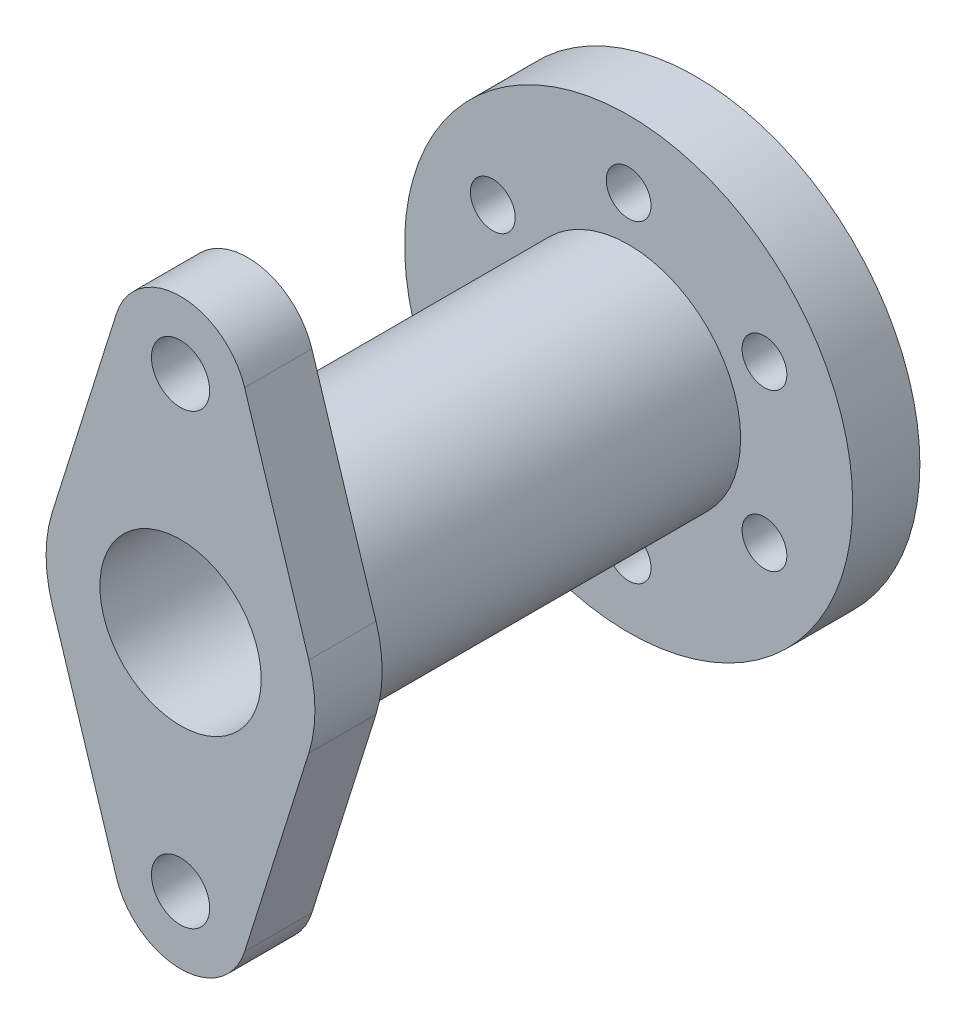
ISO-10303-21;
HEADER;
FILE_DESCRIPTION(('STEP AP214'),'2;1');
FILE_NAME('part.step','',(''),(''),'','','');
FILE_SCHEMA(('AUTOMOTIVE_DESIGN { 1 0 10303 214 1 1 1 1 }'));
ENDSEC;
DATA;
#1=APPLICATION_CONTEXT('core data for automotive mechanical design processes');
#2=APPLICATION_PROTOCOL_DEFINITION('international standard','automotive_design',2000,#1);
#3=PRODUCT_CONTEXT('',#1,'mechanical');
#4=PRODUCT('Part','Part','',(#3));
#5=PRODUCT_RELATED_PRODUCT_CATEGORY('part','',(#4));
#6=PRODUCT_DEFINITION_FORMATION('','',#4);
#7=PRODUCT_DEFINITION_CONTEXT('part definition',#1,'design');
#8=PRODUCT_DEFINITION('design','',#6,#7);
#9=PRODUCT_DEFINITION_SHAPE('','',#8);
#10=(LENGTH_UNIT() NAMED_UNIT(*) SI_UNIT(.MILLI.,.METRE.));
#11=(NAMED_UNIT(*) PLANE_ANGLE_UNIT() SI_UNIT($,.RADIAN.));
#12=(NAMED_UNIT(*) SI_UNIT($,.STERADIAN.) SOLID_ANGLE_UNIT());
#13=UNCERTAINTY_MEASURE_WITH_UNIT(LENGTH_MEASURE(1.E-05),#10,'distance_accuracy_value','');
#14=(GEOMETRIC_REPRESENTATION_CONTEXT(3) GLOBAL_UNCERTAINTY_ASSIGNED_CONTEXT((#13)) GLOBAL_UNIT_ASSIGNED_CONTEXT((#10,
#11,#12)) REPRESENTATION_CONTEXT('',''));
#15=CARTESIAN_POINT('',(0.,0.,0.));
#16=DIRECTION('',(0.,0.,1.));
#17=DIRECTION('',(1.,0.,0.));
#18=AXIS2_PLACEMENT_3D('',#15,#16,#17);
#19=CARTESIAN_POINT('',(0.,0.,15.));
#20=DIRECTION('',(0.,0.,-1.));
#21=DIRECTION('',(-1.,0.,0.));
#22=AXIS2_PLACEMENT_3D('',#19,#20,#21);
#23=CYLINDRICAL_SURFACE('',#22,50.);
#24=CARTESIAN_POINT('',(0.,0.,15.));
#25=DIRECTION('',(0.,0.,1.));
#26=DIRECTION('',(1.,0.,0.));
#27=AXIS2_PLACEMENT_3D('',#24,#25,#26);
#28=CIRCLE('',#27,50.);
#29=CARTESIAN_POINT('',(50.,0.,15.));
#30=VERTEX_POINT('',#29);
#31=EDGE_CURVE('E11',#30,#30,#28,.T.);
#32=ORIENTED_EDGE('',*,*,#31,.F.);
#33=EDGE_LOOP('',(#32));
#34=FACE_BOUND('',#33,.T.);
#35=CARTESIAN_POINT('',(0.,0.,0.));
#36=DIRECTION('',(0.,0.,1.));
#37=DIRECTION('',(1.,0.,0.));
#38=AXIS2_PLACEMENT_3D('',#35,#36,#37);
#39=CIRCLE('',#38,50.);
#40=CARTESIAN_POINT('',(50.,0.,0.));
#41=VERTEX_POINT('',#40);
#42=EDGE_CURVE('E48',#41,#41,#39,.T.);
#43=ORIENTED_EDGE('',*,*,#42,.T.);
#44=EDGE_LOOP('',(#43));
#45=FACE_BOUND('',#44,.T.);
#46=ADVANCED_FACE('F44',(#34,#45),#23,.T.);
#47=CARTESIAN_POINT('',(0.,0.,15.));
#48=DIRECTION('',(0.,0.,1.));
#49=DIRECTION('',(1.,0.,0.));
#50=AXIS2_PLACEMENT_3D('',#47,#48,#49);
#51=PLANE('',#50);
#52=CARTESIAN_POINT('',(0.,0.,15.));
#53=DIRECTION('',(0.,0.,1.));
#54=DIRECTION('',(1.,0.,0.));
#55=AXIS2_PLACEMENT_3D('',#52,#53,#54);
#56=CIRCLE('',#55,25.);
#57=CARTESIAN_POINT('',(25.,0.,15.));
#58=VERTEX_POINT('',#57);
#59=EDGE_CURVE('E175',#58,#58,#56,.T.);
#60=ORIENTED_EDGE('',*,*,#59,.F.);
#61=EDGE_LOOP('',(#60));
#62=FACE_BOUND('',#61,.T.);
#63=CARTESIAN_POINT('',(0.,-35.,15.));
#64=DIRECTION('',(0.,0.,1.));
#65=DIRECTION('',(1.,0.,0.));
#66=AXIS2_PLACEMENT_3D('',#63,#64,#65);
#67=CIRCLE('',#66,5.);
#68=CARTESIAN_POINT('',(5.,-35.,15.));
#69=VERTEX_POINT('',#68);
#70=EDGE_CURVE('E176',#69,#69,#67,.T.);
#71=ORIENTED_EDGE('',*,*,#70,.F.);
#72=EDGE_LOOP('',(#71));
#73=FACE_BOUND('',#72,.T.);
#74=CARTESIAN_POINT('',(30.3108891324553,-17.5000000000001,15.));
#75=DIRECTION('',(0.,0.,1.));
#76=DIRECTION('',(1.,0.,0.));
#77=AXIS2_PLACEMENT_3D('',#74,#75,#76);
#78=CIRCLE('',#77,5.00000000000004);
#79=CARTESIAN_POINT('',(35.3108891324554,-17.5000000000001,15.));
#80=VERTEX_POINT('',#79);
#81=EDGE_CURVE('E201',#80,#80,#78,.T.);
#82=ORIENTED_EDGE('',*,*,#81,.F.);
#83=EDGE_LOOP('',(#82));
#84=FACE_BOUND('',#83,.T.);
#85=CARTESIAN_POINT('',(-30.3108891324553,-17.5,15.));
#86=DIRECTION('',(0.,0.,1.));
#87=DIRECTION('',(1.,0.,0.));
#88=AXIS2_PLACEMENT_3D('',#85,#86,#87);
#89=CIRCLE('',#88,5.);
#90=CARTESIAN_POINT('',(-25.3108891324553,-17.5,15.));
#91=VERTEX_POINT('',#90);
#92=EDGE_CURVE('E192',#91,#91,#89,.T.);
#93=ORIENTED_EDGE('',*,*,#92,.F.);
#94=EDGE_LOOP('',(#93));
#95=FACE_BOUND('',#94,.T.);
#96=CARTESIAN_POINT('',(30.3108891324553,17.5,15.));
#97=DIRECTION('',(0.,0.,1.));
#98=DIRECTION('',(1.,0.,0.));
#99=AXIS2_PLACEMENT_3D('',#96,#97,#98);
#100=CIRCLE('',#99,5.);
#101=CARTESIAN_POINT('',(35.3108891324553,17.5,15.));
#102=VERTEX_POINT('',#101);
#103=EDGE_CURVE('E186',#102,#102,#100,.T.);
#104=ORIENTED_EDGE('',*,*,#103,.F.);
#105=EDGE_LOOP('',(#104));
#106=FACE_BOUND('',#105,.T.);
#107=CARTESIAN_POINT('',(0.,35.,15.));
#108=DIRECTION('',(0.,0.,1.));
#109=DIRECTION('',(1.,0.,0.));
#110=AXIS2_PLACEMENT_3D('',#107,#108,#109);
#111=CIRCLE('',#110,5.);
#112=CARTESIAN_POINT('',(5.,35.,15.));
#113=VERTEX_POINT('',#112);
#114=EDGE_CURVE('E182',#113,#113,#111,.T.);
#115=ORIENTED_EDGE('',*,*,#114,.F.);
#116=EDGE_LOOP('',(#115));
#117=FACE_BOUND('',#116,.T.);
#118=CARTESIAN_POINT('',(-30.3108891324553,17.5000000000001,15.));
#119=DIRECTION('',(0.,0.,1.));
#120=DIRECTION('',(1.,0.,0.));
#121=AXIS2_PLACEMENT_3D('',#118,#119,#120);
#122=CIRCLE('',#121,4.99999999999997);
#123=CARTESIAN_POINT('',(-25.3108891324554,17.5000000000001,15.));
#124=VERTEX_POINT('',#123);
#125=EDGE_CURVE('E185',#124,#124,#122,.T.);
#126=ORIENTED_EDGE('',*,*,#125,.F.);
#127=EDGE_LOOP('',(#126));
#128=FACE_BOUND('',#127,.T.);
#129=ORIENTED_EDGE('',*,*,#31,.T.);
#130=EDGE_LOOP('',(#129));
#131=FACE_BOUND('',#130,.T.);
#132=ADVANCED_FACE('F220',(#62,#73,#84,#95,#106,#117,#128,#131),#51,.T.);
#133=CARTESIAN_POINT('',(0.,0.,0.));
#134=DIRECTION('',(0.,0.,1.));
#135=DIRECTION('',(1.,0.,0.));
#136=AXIS2_PLACEMENT_3D('',#133,#134,#135);
#137=PLANE('',#136);
#138=CARTESIAN_POINT('',(0.,0.,0.));
#139=DIRECTION('',(0.,0.,1.));
#140=DIRECTION('',(1.,0.,0.));
#141=AXIS2_PLACEMENT_3D('',#138,#139,#140);
#142=CIRCLE('',#141,14.);
#143=CARTESIAN_POINT('',(14.,0.,0.));
#144=VERTEX_POINT('',#143);
#145=EDGE_CURVE('E318',#144,#144,#142,.T.);
#146=ORIENTED_EDGE('',*,*,#145,.T.);
#147=EDGE_LOOP('',(#146));
#148=FACE_BOUND('',#147,.T.);
#149=CARTESIAN_POINT('',(0.,-35.,0.));
#150=DIRECTION('',(0.,0.,1.));
#151=DIRECTION('',(1.,0.,0.));
#152=AXIS2_PLACEMENT_3D('',#149,#150,#151);
#153=CIRCLE('',#152,5.);
#154=CARTESIAN_POINT('',(5.,-35.,0.));
#155=VERTEX_POINT('',#154);
#156=EDGE_CURVE('E202',#155,#155,#153,.T.);
#157=ORIENTED_EDGE('',*,*,#156,.T.);
#158=EDGE_LOOP('',(#157));
#159=FACE_BOUND('',#158,.T.);
#160=CARTESIAN_POINT('',(30.3108891324553,-17.5000000000001,0.));
#161=DIRECTION('',(0.,0.,1.));
#162=DIRECTION('',(1.,0.,0.));
#163=AXIS2_PLACEMENT_3D('',#160,#161,#162);
#164=CIRCLE('',#163,5.00000000000004);
#165=CARTESIAN_POINT('',(35.3108891324554,-17.5000000000001,0.));
#166=VERTEX_POINT('',#165);
#167=EDGE_CURVE('E196',#166,#166,#164,.T.);
#168=ORIENTED_EDGE('',*,*,#167,.T.);
#169=EDGE_LOOP('',(#168));
#170=FACE_BOUND('',#169,.T.);
#171=CARTESIAN_POINT('',(-30.3108891324553,-17.5,0.));
#172=DIRECTION('',(0.,0.,1.));
#173=DIRECTION('',(1.,0.,0.));
#174=AXIS2_PLACEMENT_3D('',#171,#172,#173);
#175=CIRCLE('',#174,5.);
#176=CARTESIAN_POINT('',(-25.3108891324553,-17.5,0.));
#177=VERTEX_POINT('',#176);
#178=EDGE_CURVE('E191',#177,#177,#175,.T.);
#179=ORIENTED_EDGE('',*,*,#178,.T.);
#180=EDGE_LOOP('',(#179));
#181=FACE_BOUND('',#180,.T.);
#182=CARTESIAN_POINT('',(30.3108891324553,17.5,0.));
#183=DIRECTION('',(0.,0.,1.));
#184=DIRECTION('',(1.,0.,0.));
#185=AXIS2_PLACEMENT_3D('',#182,#183,#184);
#186=CIRCLE('',#185,5.);
#187=CARTESIAN_POINT('',(35.3108891324553,17.5,0.));
#188=VERTEX_POINT('',#187);
#189=EDGE_CURVE('E187',#188,#188,#186,.T.);
#190=ORIENTED_EDGE('',*,*,#189,.T.);
#191=EDGE_LOOP('',(#190));
#192=FACE_BOUND('',#191,.T.);
#193=CARTESIAN_POINT('',(0.,35.,0.));
#194=DIRECTION('',(0.,0.,1.));
#195=DIRECTION('',(1.,0.,0.));
#196=AXIS2_PLACEMENT_3D('',#193,#194,#195);
#197=CIRCLE('',#196,5.);
#198=CARTESIAN_POINT('',(5.,35.,0.));
#199=VERTEX_POINT('',#198);
#200=EDGE_CURVE('E177',#199,#199,#197,.T.);
#201=ORIENTED_EDGE('',*,*,#200,.T.);
#202=EDGE_LOOP('',(#201));
#203=FACE_BOUND('',#202,.T.);
#204=CARTESIAN_POINT('',(-30.3108891324553,17.5000000000001,0.));
#205=DIRECTION('',(0.,0.,1.));
#206=DIRECTION('',(1.,0.,0.));
#207=AXIS2_PLACEMENT_3D('',#204,#205,#206);
#208=CIRCLE('',#207,4.99999999999997);
#209=CARTESIAN_POINT('',(-25.3108891324554,17.5000000000001,0.));
#210=VERTEX_POINT('',#209);
#211=EDGE_CURVE('E209',#210,#210,#208,.T.);
#212=ORIENTED_EDGE('',*,*,#211,.T.);
#213=EDGE_LOOP('',(#212));
#214=FACE_BOUND('',#213,.T.);
#215=ORIENTED_EDGE('',*,*,#42,.F.);
#216=EDGE_LOOP('',(#215));
#217=FACE_BOUND('',#216,.T.);
#218=ADVANCED_FACE('F217',(#148,#159,#170,#181,#192,#203,#214,#217),#137,.F.);
#219=CARTESIAN_POINT('',(-30.3108891324553,17.5000000000001,0.));
#220=DIRECTION('',(0.,0.,1.));
#221=DIRECTION('',(1.,0.,0.));
#222=AXIS2_PLACEMENT_3D('',#219,#220,#221);
#223=CYLINDRICAL_SURFACE('',#222,4.99999999999997);
#224=ORIENTED_EDGE('',*,*,#211,.F.);
#225=EDGE_LOOP('',(#224));
#226=FACE_BOUND('',#225,.T.);
#227=ORIENTED_EDGE('',*,*,#125,.T.);
#228=EDGE_LOOP('',(#227));
#229=FACE_BOUND('',#228,.T.);
#230=ADVANCED_FACE('F212',(#226,#229),#223,.F.);
#231=CARTESIAN_POINT('',(0.,35.,0.));
#232=DIRECTION('',(0.,0.,1.));
#233=DIRECTION('',(1.,0.,0.));
#234=AXIS2_PLACEMENT_3D('',#231,#232,#233);
#235=CYLINDRICAL_SURFACE('',#234,5.);
#236=ORIENTED_EDGE('',*,*,#200,.F.);
#237=EDGE_LOOP('',(#236));
#238=FACE_BOUND('',#237,.T.);
#239=ORIENTED_EDGE('',*,*,#114,.T.);
#240=EDGE_LOOP('',(#239));
#241=FACE_BOUND('',#240,.T.);
#242=ADVANCED_FACE('F236',(#238,#241),#235,.F.);
#243=CARTESIAN_POINT('',(30.3108891324553,17.5,0.));
#244=DIRECTION('',(0.,0.,1.));
#245=DIRECTION('',(1.,0.,0.));
#246=AXIS2_PLACEMENT_3D('',#243,#244,#245);
#247=CYLINDRICAL_SURFACE('',#246,5.);
#248=ORIENTED_EDGE('',*,*,#189,.F.);
#249=EDGE_LOOP('',(#248));
#250=FACE_BOUND('',#249,.T.);
#251=ORIENTED_EDGE('',*,*,#103,.T.);
#252=EDGE_LOOP('',(#251));
#253=FACE_BOUND('',#252,.T.);
#254=ADVANCED_FACE('F251',(#250,#253),#247,.F.);
#255=CARTESIAN_POINT('',(-30.3108891324553,-17.5,0.));
#256=DIRECTION('',(0.,0.,1.));
#257=DIRECTION('',(1.,0.,0.));
#258=AXIS2_PLACEMENT_3D('',#255,#256,#257);
#259=CYLINDRICAL_SURFACE('',#258,5.);
#260=ORIENTED_EDGE('',*,*,#178,.F.);
#261=EDGE_LOOP('',(#260));
#262=FACE_BOUND('',#261,.T.);
#263=ORIENTED_EDGE('',*,*,#92,.T.);
#264=EDGE_LOOP('',(#263));
#265=FACE_BOUND('',#264,.T.);
#266=ADVANCED_FACE('F249',(#262,#265),#259,.F.);
#267=CARTESIAN_POINT('',(30.3108891324553,-17.5000000000001,0.));
#268=DIRECTION('',(0.,0.,1.));
#269=DIRECTION('',(1.,0.,0.));
#270=AXIS2_PLACEMENT_3D('',#267,#268,#269);
#271=CYLINDRICAL_SURFACE('',#270,5.00000000000004);
#272=ORIENTED_EDGE('',*,*,#167,.F.);
#273=EDGE_LOOP('',(#272));
#274=FACE_BOUND('',#273,.T.);
#275=ORIENTED_EDGE('',*,*,#81,.T.);
#276=EDGE_LOOP('',(#275));
#277=FACE_BOUND('',#276,.T.);
#278=ADVANCED_FACE('F246',(#274,#277),#271,.F.);
#279=CARTESIAN_POINT('',(0.,-35.,0.));
#280=DIRECTION('',(0.,0.,1.));
#281=DIRECTION('',(1.,0.,0.));
#282=AXIS2_PLACEMENT_3D('',#279,#280,#281);
#283=CYLINDRICAL_SURFACE('',#282,5.);
#284=ORIENTED_EDGE('',*,*,#156,.F.);
#285=EDGE_LOOP('',(#284));
#286=FACE_BOUND('',#285,.T.);
#287=ORIENTED_EDGE('',*,*,#70,.T.);
#288=EDGE_LOOP('',(#287));
#289=FACE_BOUND('',#288,.T.);
#290=ADVANCED_FACE('F245',(#286,#289),#283,.F.);
#291=CARTESIAN_POINT('',(0.,0.,100.));
#292=DIRECTION('',(0.,0.,-1.));
#293=DIRECTION('',(-1.,0.,0.));
#294=AXIS2_PLACEMENT_3D('',#291,#292,#293);
#295=CYLINDRICAL_SURFACE('',#294,25.);
#296=CARTESIAN_POINT('',(0.,0.,100.));
#297=DIRECTION('',(0.,0.,1.));
#298=DIRECTION('',(1.,0.,0.));
#299=AXIS2_PLACEMENT_3D('',#296,#297,#298);
#300=CIRCLE('',#299,25.);
#301=CARTESIAN_POINT('',(25.,0.,100.));
#302=VERTEX_POINT('',#301);
#303=EDGE_CURVE('E173',#302,#302,#300,.T.);
#304=ORIENTED_EDGE('',*,*,#303,.F.);
#305=EDGE_LOOP('',(#304));
#306=FACE_BOUND('',#305,.T.);
#307=ORIENTED_EDGE('',*,*,#59,.T.);
#308=EDGE_LOOP('',(#307));
#309=FACE_BOUND('',#308,.T.);
#310=ADVANCED_FACE('F244',(#306,#309),#295,.T.);
#311=CARTESIAN_POINT('',(0.,0.,115.));
#312=DIRECTION('',(0.,0.,-1.));
#313=DIRECTION('',(-1.,0.,0.));
#314=AXIS2_PLACEMENT_3D('',#311,#312,#313);
#315=CYLINDRICAL_SURFACE('',#314,30.);
#316=CARTESIAN_POINT('',(0.,0.,100.));
#317=DIRECTION('',(0.,0.,1.));
#318=DIRECTION('',(1.,0.,0.));
#319=AXIS2_PLACEMENT_3D('',#316,#317,#318);
#320=CIRCLE('',#319,30.);
#321=CARTESIAN_POINT('',(-28.6181760425107,8.99999999999249,100.));
#322=VERTEX_POINT('',#321);
#323=CARTESIAN_POINT('',(-28.6181760425107,-8.9999999999925,100.));
#324=VERTEX_POINT('',#323);
#325=EDGE_CURVE('E145',#322,#324,#320,.T.);
#326=ORIENTED_EDGE('',*,*,#325,.T.);
#327=DIRECTION('',(0.,0.,-1.));
#328=VECTOR('',#327,1.);
#329=CARTESIAN_POINT('',(-28.6181760425107,-8.9999999999925,115.));
#330=LINE('',#329,#328);
#331=CARTESIAN_POINT('',(-28.6181760425107,-8.9999999999925,115.));
#332=VERTEX_POINT('',#331);
#333=EDGE_CURVE('E167',#332,#324,#330,.T.);
#334=ORIENTED_EDGE('',*,*,#333,.F.);
#335=CARTESIAN_POINT('',(0.,0.,115.));
#336=DIRECTION('',(0.,0.,1.));
#337=DIRECTION('',(1.,0.,0.));
#338=AXIS2_PLACEMENT_3D('',#335,#336,#337);
#339=CIRCLE('',#338,30.);
#340=CARTESIAN_POINT('',(-28.6181760425107,8.99999999999249,115.));
#341=VERTEX_POINT('',#340);
#342=EDGE_CURVE('E160',#341,#332,#339,.T.);
#343=ORIENTED_EDGE('',*,*,#342,.F.);
#344=DIRECTION('',(0.,0.,-1.));
#345=VECTOR('',#344,1.);
#346=CARTESIAN_POINT('',(-28.6181760425107,8.99999999999249,115.));
#347=LINE('',#346,#345);
#348=EDGE_CURVE('E138',#341,#322,#347,.T.);
#349=ORIENTED_EDGE('',*,*,#348,.T.);
#350=EDGE_LOOP('',(#326,#334,#343,#349));
#351=FACE_BOUND('',#350,.T.);
#352=ADVANCED_FACE('F261',(#351),#315,.T.);
#353=CARTESIAN_POINT('',(-28.6181760425107,-8.9999999999925,115.));
#354=DIRECTION('',(0.953939201417024,0.29999999999975,0.));
#355=DIRECTION('',(-0.29999999999975,0.953939201417024,0.));
#356=AXIS2_PLACEMENT_3D('',#353,#354,#355);
#357=PLANE('',#356);
#358=DIRECTION('',(0.29999999999975,-0.953939201417024,0.));
#359=VECTOR('',#358,1.);
#360=CARTESIAN_POINT('',(-28.6181760425107,-8.9999999999925,100.));
#361=LINE('',#360,#359);
#362=CARTESIAN_POINT('',(-14.3090880212673,-54.5,100.));
#363=VERTEX_POINT('',#362);
#364=EDGE_CURVE('E143',#324,#363,#361,.T.);
#365=ORIENTED_EDGE('',*,*,#364,.T.);
#366=DIRECTION('',(0.,0.,-1.));
#367=VECTOR('',#366,1.);
#368=CARTESIAN_POINT('',(-14.3090880212673,-54.5,115.));
#369=LINE('',#368,#367);
#370=CARTESIAN_POINT('',(-14.3090880212673,-54.5,115.));
#371=VERTEX_POINT('',#370);
#372=EDGE_CURVE('E170',#371,#363,#369,.T.);
#373=ORIENTED_EDGE('',*,*,#372,.F.);
#374=DIRECTION('',(0.29999999999975,-0.953939201417024,0.));
#375=VECTOR('',#374,1.);
#376=CARTESIAN_POINT('',(-28.6181760425107,-8.9999999999925,115.));
#377=LINE('',#376,#375);
#378=EDGE_CURVE('E102',#332,#371,#377,.T.);
#379=ORIENTED_EDGE('',*,*,#378,.F.);
#380=ORIENTED_EDGE('',*,*,#333,.T.);
#381=EDGE_LOOP('',(#365,#373,#379,#380));
#382=FACE_BOUND('',#381,.T.);
#383=ADVANCED_FACE('F270',(#382),#357,.F.);
#384=CARTESIAN_POINT('',(0.,-50.,115.));
#385=DIRECTION('',(0.,0.,-1.));
#386=DIRECTION('',(-1.,0.,0.));
#387=AXIS2_PLACEMENT_3D('',#384,#385,#386);
#388=CYLINDRICAL_SURFACE('',#387,15.0000000000125);
#389=CARTESIAN_POINT('',(0.,-50.,100.));
#390=DIRECTION('',(0.,0.,1.));
#391=DIRECTION('',(1.,0.,0.));
#392=AXIS2_PLACEMENT_3D('',#389,#390,#391);
#393=CIRCLE('',#392,15.0000000000125);
#394=CARTESIAN_POINT('',(14.3090880212673,-54.5,100.));
#395=VERTEX_POINT('',#394);
#396=EDGE_CURVE('E150',#363,#395,#393,.T.);
#397=ORIENTED_EDGE('',*,*,#396,.T.);
#398=DIRECTION('',(0.,0.,-1.));
#399=VECTOR('',#398,1.);
#400=CARTESIAN_POINT('',(14.3090880212673,-54.5,115.));
#401=LINE('',#400,#399);
#402=CARTESIAN_POINT('',(14.3090880212673,-54.5,115.));
#403=VERTEX_POINT('',#402);
#404=EDGE_CURVE('E165',#403,#395,#401,.T.);
#405=ORIENTED_EDGE('',*,*,#404,.F.);
#406=CARTESIAN_POINT('',(0.,-50.,115.));
#407=DIRECTION('',(0.,0.,1.));
#408=DIRECTION('',(1.,0.,0.));
#409=AXIS2_PLACEMENT_3D('',#406,#407,#408);
#410=CIRCLE('',#409,15.0000000000125);
#411=EDGE_CURVE('E348',#371,#403,#410,.T.);
#412=ORIENTED_EDGE('',*,*,#411,.F.);
#413=ORIENTED_EDGE('',*,*,#372,.T.);
#414=EDGE_LOOP('',(#397,#405,#412,#413));
#415=FACE_BOUND('',#414,.T.);
#416=ADVANCED_FACE('F272',(#415),#388,.T.);
#417=CARTESIAN_POINT('',(14.3090880212673,-54.5,115.));
#418=DIRECTION('',(-0.953939201417024,0.29999999999975,0.));
#419=DIRECTION('',(-0.29999999999975,-0.953939201417024,0.));
#420=AXIS2_PLACEMENT_3D('',#417,#418,#419);
#421=PLANE('',#420);
#422=DIRECTION('',(0.29999999999975,0.953939201417024,0.));
#423=VECTOR('',#422,1.);
#424=CARTESIAN_POINT('',(14.3090880212673,-54.5,100.));
#425=LINE('',#424,#423);
#426=CARTESIAN_POINT('',(28.6181760425107,-8.99999999999251,100.));
#427=VERTEX_POINT('',#426);
#428=EDGE_CURVE('E147',#395,#427,#425,.T.);
#429=ORIENTED_EDGE('',*,*,#428,.T.);
#430=DIRECTION('',(0.,0.,-1.));
#431=VECTOR('',#430,1.);
#432=CARTESIAN_POINT('',(28.6181760425107,-8.99999999999251,115.));
#433=LINE('',#432,#431);
#434=CARTESIAN_POINT('',(28.6181760425107,-8.99999999999251,115.));
#435=VERTEX_POINT('',#434);
#436=EDGE_CURVE('E163',#435,#427,#433,.T.);
#437=ORIENTED_EDGE('',*,*,#436,.F.);
#438=DIRECTION('',(0.29999999999975,0.953939201417024,0.));
#439=VECTOR('',#438,1.);
#440=CARTESIAN_POINT('',(14.3090880212673,-54.5,115.));
#441=LINE('',#440,#439);
#442=EDGE_CURVE('E346',#403,#435,#441,.T.);
#443=ORIENTED_EDGE('',*,*,#442,.F.);
#444=ORIENTED_EDGE('',*,*,#404,.T.);
#445=EDGE_LOOP('',(#429,#437,#443,#444));
#446=FACE_BOUND('',#445,.T.);
#447=ADVANCED_FACE('F274',(#446),#421,.F.);
#448=CARTESIAN_POINT('',(0.,0.,115.));
#449=DIRECTION('',(0.,0.,-1.));
#450=DIRECTION('',(-1.,0.,0.));
#451=AXIS2_PLACEMENT_3D('',#448,#449,#450);
#452=CYLINDRICAL_SURFACE('',#451,30.);
#453=CARTESIAN_POINT('',(0.,0.,100.));
#454=DIRECTION('',(0.,0.,1.));
#455=DIRECTION('',(1.,0.,0.));
#456=AXIS2_PLACEMENT_3D('',#453,#454,#455);
#457=CIRCLE('',#456,30.);
#458=CARTESIAN_POINT('',(28.6181760425107,8.99999999999249,100.));
#459=VERTEX_POINT('',#458);
#460=EDGE_CURVE('E155',#427,#459,#457,.T.);
#461=ORIENTED_EDGE('',*,*,#460,.T.);
#462=DIRECTION('',(0.,0.,-1.));
#463=VECTOR('',#462,1.);
#464=CARTESIAN_POINT('',(28.6181760425107,8.99999999999249,115.));
#465=LINE('',#464,#463);
#466=CARTESIAN_POINT('',(28.6181760425107,8.99999999999249,115.));
#467=VERTEX_POINT('',#466);
#468=EDGE_CURVE('E131',#467,#459,#465,.T.);
#469=ORIENTED_EDGE('',*,*,#468,.F.);
#470=CARTESIAN_POINT('',(0.,0.,115.));
#471=DIRECTION('',(0.,0.,1.));
#472=DIRECTION('',(1.,0.,0.));
#473=AXIS2_PLACEMENT_3D('',#470,#471,#472);
#474=CIRCLE('',#473,30.);
#475=EDGE_CURVE('E121',#435,#467,#474,.T.);
#476=ORIENTED_EDGE('',*,*,#475,.F.);
#477=ORIENTED_EDGE('',*,*,#436,.T.);
#478=EDGE_LOOP('',(#461,#469,#476,#477));
#479=FACE_BOUND('',#478,.T.);
#480=ADVANCED_FACE('F280',(#479),#452,.T.);
#481=CARTESIAN_POINT('',(14.3090880212673,54.5,115.));
#482=DIRECTION('',(-0.953939201417024,-0.29999999999975,0.));
#483=DIRECTION('',(0.29999999999975,-0.953939201417024,0.));
#484=AXIS2_PLACEMENT_3D('',#481,#482,#483);
#485=PLANE('',#484);
#486=DIRECTION('',(-0.29999999999975,0.953939201417024,0.));
#487=VECTOR('',#486,1.);
#488=CARTESIAN_POINT('',(14.3090880212673,54.5,100.));
#489=LINE('',#488,#487);
#490=CARTESIAN_POINT('',(14.3090880212673,54.5,100.));
#491=VERTEX_POINT('',#490);
#492=EDGE_CURVE('E135',#459,#491,#489,.T.);
#493=ORIENTED_EDGE('',*,*,#492,.T.);
#494=DIRECTION('',(0.,0.,-1.));
#495=VECTOR('',#494,1.);
#496=CARTESIAN_POINT('',(14.3090880212673,54.5,115.));
#497=LINE('',#496,#495);
#498=CARTESIAN_POINT('',(14.3090880212673,54.5,115.));
#499=VERTEX_POINT('',#498);
#500=EDGE_CURVE('E128',#499,#491,#497,.T.);
#501=ORIENTED_EDGE('',*,*,#500,.F.);
#502=DIRECTION('',(-0.29999999999975,0.953939201417024,0.));
#503=VECTOR('',#502,1.);
#504=CARTESIAN_POINT('',(14.3090880212673,54.5,115.));
#505=LINE('',#504,#503);
#506=EDGE_CURVE('E117',#467,#499,#505,.T.);
#507=ORIENTED_EDGE('',*,*,#506,.F.);
#508=ORIENTED_EDGE('',*,*,#468,.T.);
#509=EDGE_LOOP('',(#493,#501,#507,#508));
#510=FACE_BOUND('',#509,.T.);
#511=ADVANCED_FACE('F127',(#510),#485,.F.);
#512=CARTESIAN_POINT('',(0.,50.,115.));
#513=DIRECTION('',(0.,0.,-1.));
#514=DIRECTION('',(-1.,0.,0.));
#515=AXIS2_PLACEMENT_3D('',#512,#513,#514);
#516=CYLINDRICAL_SURFACE('',#515,15.0000000000125);
#517=CARTESIAN_POINT('',(0.,50.,100.));
#518=DIRECTION('',(0.,0.,1.));
#519=DIRECTION('',(1.,0.,0.));
#520=AXIS2_PLACEMENT_3D('',#517,#518,#519);
#521=CIRCLE('',#520,15.0000000000125);
#522=CARTESIAN_POINT('',(-14.3090880212673,54.5,100.));
#523=VERTEX_POINT('',#522);
#524=EDGE_CURVE('E87',#491,#523,#521,.T.);
#525=ORIENTED_EDGE('',*,*,#524,.T.);
#526=DIRECTION('',(0.,0.,-1.));
#527=VECTOR('',#526,1.);
#528=CARTESIAN_POINT('',(-14.3090880212673,54.5,115.));
#529=LINE('',#528,#527);
#530=CARTESIAN_POINT('',(-14.3090880212673,54.5,115.));
#531=VERTEX_POINT('',#530);
#532=EDGE_CURVE('E134',#531,#523,#529,.T.);
#533=ORIENTED_EDGE('',*,*,#532,.F.);
#534=CARTESIAN_POINT('',(0.,50.,115.));
#535=DIRECTION('',(0.,0.,1.));
#536=DIRECTION('',(1.,0.,0.));
#537=AXIS2_PLACEMENT_3D('',#534,#535,#536);
#538=CIRCLE('',#537,15.0000000000125);
#539=EDGE_CURVE('E125',#499,#531,#538,.T.);
#540=ORIENTED_EDGE('',*,*,#539,.F.);
#541=ORIENTED_EDGE('',*,*,#500,.T.);
#542=EDGE_LOOP('',(#525,#533,#540,#541));
#543=FACE_BOUND('',#542,.T.);
#544=ADVANCED_FACE('F136',(#543),#516,.T.);
#545=CARTESIAN_POINT('',(-28.6181760425107,8.99999999999249,115.));
#546=DIRECTION('',(0.953939201417024,-0.29999999999975,0.));
#547=DIRECTION('',(0.29999999999975,0.953939201417024,0.));
#548=AXIS2_PLACEMENT_3D('',#545,#546,#547);
#549=PLANE('',#548);
#550=DIRECTION('',(-0.29999999999975,-0.953939201417024,0.));
#551=VECTOR('',#550,1.);
#552=CARTESIAN_POINT('',(-28.6181760425107,8.99999999999249,100.));
#553=LINE('',#552,#551);
#554=EDGE_CURVE('E98',#523,#322,#553,.T.);
#555=ORIENTED_EDGE('',*,*,#554,.T.);
#556=ORIENTED_EDGE('',*,*,#348,.F.);
#557=DIRECTION('',(-0.29999999999975,-0.953939201417024,0.));
#558=VECTOR('',#557,1.);
#559=CARTESIAN_POINT('',(-28.6181760425107,8.99999999999249,115.));
#560=LINE('',#559,#558);
#561=EDGE_CURVE('E64',#531,#341,#560,.T.);
#562=ORIENTED_EDGE('',*,*,#561,.F.);
#563=ORIENTED_EDGE('',*,*,#532,.T.);
#564=EDGE_LOOP('',(#555,#556,#562,#563));
#565=FACE_BOUND('',#564,.T.);
#566=ADVANCED_FACE('F290',(#565),#549,.F.);
#567=CARTESIAN_POINT('',(0.,0.,115.));
#568=DIRECTION('',(0.,0.,1.));
#569=DIRECTION('',(1.,0.,0.));
#570=AXIS2_PLACEMENT_3D('',#567,#568,#569);
#571=PLANE('',#570);
#572=CARTESIAN_POINT('',(0.,0.,115.));
#573=DIRECTION('',(0.,0.,1.));
#574=DIRECTION('',(1.,0.,0.));
#575=AXIS2_PLACEMENT_3D('',#572,#573,#574);
#576=CIRCLE('',#575,18.);
#577=CARTESIAN_POINT('',(18.,0.,115.));
#578=VERTEX_POINT('',#577);
#579=EDGE_CURVE('E322',#578,#578,#576,.T.);
#580=ORIENTED_EDGE('',*,*,#579,.F.);
#581=EDGE_LOOP('',(#580));
#582=FACE_BOUND('',#581,.T.);
#583=CARTESIAN_POINT('',(0.,50.,115.));
#584=DIRECTION('',(0.,0.,1.));
#585=DIRECTION('',(1.,0.,0.));
#586=AXIS2_PLACEMENT_3D('',#583,#584,#585);
#587=CIRCLE('',#586,6.5);
#588=CARTESIAN_POINT('',(6.5,50.,115.));
#589=VERTEX_POINT('',#588);
#590=EDGE_CURVE('E337',#589,#589,#587,.T.);
#591=ORIENTED_EDGE('',*,*,#590,.F.);
#592=EDGE_LOOP('',(#591));
#593=FACE_BOUND('',#592,.T.);
#594=CARTESIAN_POINT('',(0.,-50.,115.));
#595=DIRECTION('',(0.,0.,1.));
#596=DIRECTION('',(1.,0.,0.));
#597=AXIS2_PLACEMENT_3D('',#594,#595,#596);
#598=CIRCLE('',#597,6.5);
#599=CARTESIAN_POINT('',(6.5,-50.,115.));
#600=VERTEX_POINT('',#599);
#601=EDGE_CURVE('E331',#600,#600,#598,.T.);
#602=ORIENTED_EDGE('',*,*,#601,.F.);
#603=EDGE_LOOP('',(#602));
#604=FACE_BOUND('',#603,.T.);
#605=ORIENTED_EDGE('',*,*,#342,.T.);
#606=ORIENTED_EDGE('',*,*,#378,.T.);
#607=ORIENTED_EDGE('',*,*,#411,.T.);
#608=ORIENTED_EDGE('',*,*,#442,.T.);
#609=ORIENTED_EDGE('',*,*,#475,.T.);
#610=ORIENTED_EDGE('',*,*,#506,.T.);
#611=ORIENTED_EDGE('',*,*,#539,.T.);
#612=ORIENTED_EDGE('',*,*,#561,.T.);
#613=EDGE_LOOP('',(#605,#606,#607,#608,#609,#610,#611,#612));
#614=FACE_BOUND('',#613,.T.);
#615=ADVANCED_FACE('F119',(#582,#593,#604,#614),#571,.T.);
#616=CARTESIAN_POINT('',(0.,0.,100.));
#617=DIRECTION('',(0.,0.,1.));
#618=DIRECTION('',(1.,0.,0.));
#619=AXIS2_PLACEMENT_3D('',#616,#617,#618);
#620=PLANE('',#619);
#621=CARTESIAN_POINT('',(0.,50.,100.));
#622=DIRECTION('',(0.,0.,1.));
#623=DIRECTION('',(1.,0.,0.));
#624=AXIS2_PLACEMENT_3D('',#621,#622,#623);
#625=CIRCLE('',#624,6.5);
#626=CARTESIAN_POINT('',(6.5,50.,100.));
#627=VERTEX_POINT('',#626);
#628=EDGE_CURVE('E149',#627,#627,#625,.T.);
#629=ORIENTED_EDGE('',*,*,#628,.T.);
#630=EDGE_LOOP('',(#629));
#631=FACE_BOUND('',#630,.T.);
#632=CARTESIAN_POINT('',(0.,-50.,100.));
#633=DIRECTION('',(0.,0.,1.));
#634=DIRECTION('',(1.,0.,0.));
#635=AXIS2_PLACEMENT_3D('',#632,#633,#634);
#636=CIRCLE('',#635,6.5);
#637=CARTESIAN_POINT('',(6.5,-50.,100.));
#638=VERTEX_POINT('',#637);
#639=EDGE_CURVE('E339',#638,#638,#636,.T.);
#640=ORIENTED_EDGE('',*,*,#639,.T.);
#641=EDGE_LOOP('',(#640));
#642=FACE_BOUND('',#641,.T.);
#643=ORIENTED_EDGE('',*,*,#303,.T.);
#644=EDGE_LOOP('',(#643));
#645=FACE_BOUND('',#644,.T.);
#646=ORIENTED_EDGE('',*,*,#325,.F.);
#647=ORIENTED_EDGE('',*,*,#554,.F.);
#648=ORIENTED_EDGE('',*,*,#524,.F.);
#649=ORIENTED_EDGE('',*,*,#492,.F.);
#650=ORIENTED_EDGE('',*,*,#460,.F.);
#651=ORIENTED_EDGE('',*,*,#428,.F.);
#652=ORIENTED_EDGE('',*,*,#396,.F.);
#653=ORIENTED_EDGE('',*,*,#364,.F.);
#654=EDGE_LOOP('',(#646,#647,#648,#649,#650,#651,#652,#653));
#655=FACE_BOUND('',#654,.T.);
#656=ADVANCED_FACE('F289',(#631,#642,#645,#655),#620,.F.);
#657=CARTESIAN_POINT('',(0.,-50.,100.));
#658=DIRECTION('',(0.,0.,1.));
#659=DIRECTION('',(1.,0.,0.));
#660=AXIS2_PLACEMENT_3D('',#657,#658,#659);
#661=CYLINDRICAL_SURFACE('',#660,6.5);
#662=ORIENTED_EDGE('',*,*,#639,.F.);
#663=EDGE_LOOP('',(#662));
#664=FACE_BOUND('',#663,.T.);
#665=ORIENTED_EDGE('',*,*,#601,.T.);
#666=EDGE_LOOP('',(#665));
#667=FACE_BOUND('',#666,.T.);
#668=ADVANCED_FACE('F291',(#664,#667),#661,.F.);
#669=CARTESIAN_POINT('',(0.,50.,100.));
#670=DIRECTION('',(0.,0.,1.));
#671=DIRECTION('',(1.,0.,0.));
#672=AXIS2_PLACEMENT_3D('',#669,#670,#671);
#673=CYLINDRICAL_SURFACE('',#672,6.5);
#674=ORIENTED_EDGE('',*,*,#628,.F.);
#675=EDGE_LOOP('',(#674));
#676=FACE_BOUND('',#675,.T.);
#677=ORIENTED_EDGE('',*,*,#590,.T.);
#678=EDGE_LOOP('',(#677));
#679=FACE_BOUND('',#678,.T.);
#680=ADVANCED_FACE('F297',(#676,#679),#673,.F.);
#681=CARTESIAN_POINT('',(0.,0.,75.));
#682=DIRECTION('',(0.,0.,1.));
#683=DIRECTION('',(1.,0.,0.));
#684=AXIS2_PLACEMENT_3D('',#681,#682,#683);
#685=CYLINDRICAL_SURFACE('',#684,18.);
#686=CARTESIAN_POINT('',(0.,0.,75.));
#687=DIRECTION('',(0.,0.,1.));
#688=DIRECTION('',(1.,0.,0.));
#689=AXIS2_PLACEMENT_3D('',#686,#687,#688);
#690=CIRCLE('',#689,18.);
#691=CARTESIAN_POINT('',(18.,0.,75.));
#692=VERTEX_POINT('',#691);
#693=EDGE_CURVE('E326',#692,#692,#690,.T.);
#694=ORIENTED_EDGE('',*,*,#693,.F.);
#695=EDGE_LOOP('',(#694));
#696=FACE_BOUND('',#695,.T.);
#697=ORIENTED_EDGE('',*,*,#579,.T.);
#698=EDGE_LOOP('',(#697));
#699=FACE_BOUND('',#698,.T.);
#700=ADVANCED_FACE('F302',(#696,#699),#685,.F.);
#701=CARTESIAN_POINT('',(0.,0.,75.));
#702=DIRECTION('',(0.,0.,1.));
#703=DIRECTION('',(1.,0.,0.));
#704=AXIS2_PLACEMENT_3D('',#701,#702,#703);
#705=PLANE('',#704);
#706=CARTESIAN_POINT('',(0.,0.,75.));
#707=DIRECTION('',(0.,0.,1.));
#708=DIRECTION('',(1.,0.,0.));
#709=AXIS2_PLACEMENT_3D('',#706,#707,#708);
#710=CIRCLE('',#709,14.);
#711=CARTESIAN_POINT('',(14.,0.,75.));
#712=VERTEX_POINT('',#711);
#713=EDGE_CURVE('E325',#712,#712,#710,.T.);
#714=ORIENTED_EDGE('',*,*,#713,.F.);
#715=EDGE_LOOP('',(#714));
#716=FACE_BOUND('',#715,.T.);
#717=ORIENTED_EDGE('',*,*,#693,.T.);
#718=EDGE_LOOP('',(#717));
#719=FACE_BOUND('',#718,.T.);
#720=ADVANCED_FACE('F308',(#716,#719),#705,.T.);
#721=CARTESIAN_POINT('',(0.,0.,0.));
#722=DIRECTION('',(0.,0.,1.));
#723=DIRECTION('',(1.,0.,0.));
#724=AXIS2_PLACEMENT_3D('',#721,#722,#723);
#725=CYLINDRICAL_SURFACE('',#724,14.);
#726=ORIENTED_EDGE('',*,*,#145,.F.);
#727=EDGE_LOOP('',(#726));
#728=FACE_BOUND('',#727,.T.);
#729=ORIENTED_EDGE('',*,*,#713,.T.);
#730=EDGE_LOOP('',(#729));
#731=FACE_BOUND('',#730,.T.);
#732=ADVANCED_FACE('F315',(#728,#731),#725,.F.);
#733=CLOSED_SHELL('',(#46,#132,#218,#230,#242,#254,#266,#278,#290,#310,#352,#383,#416,#447,#480,
#511,#544,#566,#615,#656,#668,#680,#700,#720,#732));
#734=MANIFOLD_SOLID_BREP('B2',#733);
#735=ADVANCED_BREP_SHAPE_REPRESENTATION('',(#18,#734),#14);
#736=SHAPE_DEFINITION_REPRESENTATION(#9,#735);
ENDSEC;
END-ISO-10303-21;
